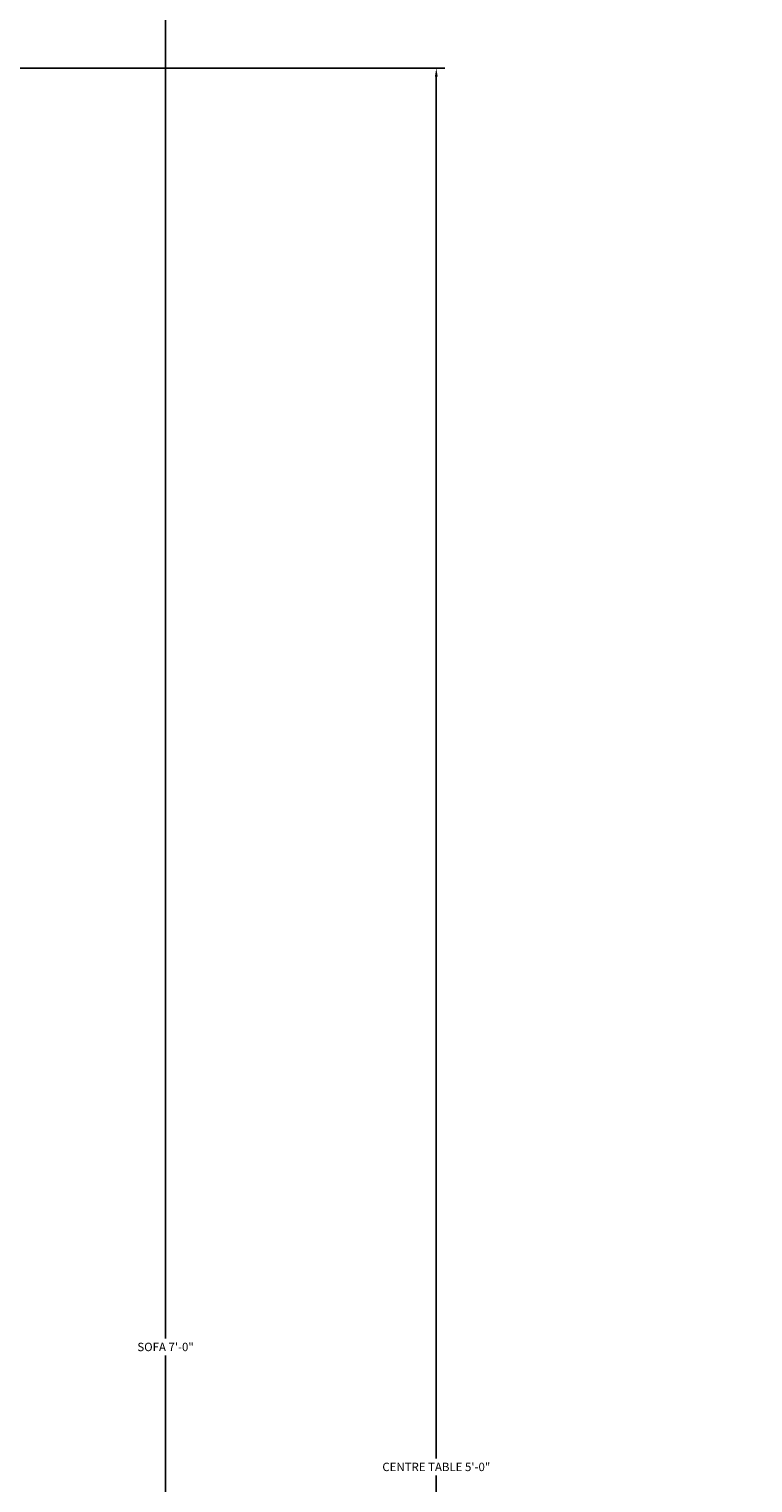
# Model space of a CAD drawing. Units: inches. Extents: x -105 to 1196, y -792 to 119.
# Tile 14 of 23: x 262 to 278, y -349 to -318. Entities that reach past the tile are written whole.
import ezdxf

# ---------------------------------------------------------------- set-up
doc = ezdxf.new("R2010")
doc.units = ezdxf.units.IN
doc.header["$MEASUREMENT"] = 0
doc.layers.add('A-ANNO-DIMS', color=2, linetype='Continuous', lineweight=18)
doc.styles.get("Standard").update_dxf_attribs({"font": 'arial.ttf'})
doc.dimstyles.get("Standard").update_dxf_attribs({"dimtxt": 0.18, "dimasz": 0.18, "dimexe": 0.18, "dimexo": 0.0625, "dimgap": 0.09, "dimtad": 0, "dimtih": 1, "dimtoh": 1, "dimdec": 1, "dimzin": 0, "dimdsep": 46, "dimlunit": 4, "dimtxsty": 'Standard', "dimcen": 0.09, "dimadec": 0, "dimazin": 0, "dimtfac": 1, "dimtdec": 1, "dimtofl": 0, "dimtmove": 0, "dimatfit": 3, "dimfxl": 1, "dimtolj": 1, "dimtzin": 0, "dimarcsym": 0})

# ---------------------------------------------------------------- blocks, each defined once
blk = doc.blocks.new('*D77')
at = {"layer": 'A-ANNO-DIMS', "color": 0, "lineweight": -2, "transparency": 16777216}
for p, q in [((277.544, -304.122), (264.827, -304.122)), ((265.007, -304.302), (265.007, -345.939)), ((265.007, -387.942), (265.007, -346.305)), ((277.544, -388.122), (264.827, -388.122))]:
    blk.add_line(p, q, dxfattribs=at)
at = {"layer": 'A-ANNO-DIMS', "color": 0, "transparency": 16777216}
for points in [[(264.977, -304.302), (265.037, -304.302), (265.007, -304.122)], [(264.977, -387.942), (265.037, -387.942), (265.007, -388.122)]]:
    blk.add_solid(points, dxfattribs=at)
at = {"layer": 'Defpoints', "color": 0, "transparency": 16777216}
for p in [(277.607, -304.122), (265.007, -388.122), (277.607, -388.122)]:
    blk.add_point(p, dxfattribs=at)
at = {"layer": 'A-ANNO-DIMS', "color": 0, "transparency": 16777216, "insert": (265.007, -346.122), "char_height": 0.18, "attachment_point": 5}
blk.add_mtext('\\A1;SOFA 7\'-0"', dxfattribs=at)
blk = doc.blocks.new('*D83')
at = {"layer": 'A-ANNO-DIMS', "color": 0, "lineweight": -2, "transparency": 16777216}
for p, q in [((261.878, -318.695), (270.995, -318.695)), ((270.815, -318.875), (270.815, -348.512)), ((270.815, -378.515), (270.815, -348.878)), ((261.878, -378.695), (270.995, -378.695))]:
    blk.add_line(p, q, dxfattribs=at)
at = {"layer": 'A-ANNO-DIMS', "color": 0, "transparency": 16777216}
for points in [[(270.785, -318.875), (270.845, -318.875), (270.815, -318.695)], [(270.785, -378.515), (270.845, -378.515), (270.815, -378.695)]]:
    blk.add_solid(points, dxfattribs=at)
at = {"layer": 'Defpoints', "color": 0, "transparency": 16777216}
for p in [(261.815, -318.695), (270.815, -318.695), (261.815, -378.695)]:
    blk.add_point(p, dxfattribs=at)
at = {"layer": 'A-ANNO-DIMS', "color": 0, "transparency": 16777216, "insert": (270.815, -348.695), "char_height": 0.18, "attachment_point": 5}
blk.add_mtext('\\A1;CENTRE TABLE 5\'-0"', dxfattribs=at)

msp = doc.modelspace()

# ---------------------------------------------------------------- dimensions: what is measured, and where the dimension line sits
at = {"layer": 'A-ANNO-DIMS'}
for base, p1, p2, angle, text, picture, middle in [((265.007, -388.122), (277.607, -304.122), (277.607, -388.122), 270, 'SOFA <>', '*D77', (265.007, -346.122)), ((270.815, -318.695), (261.815, -378.695), (261.815, -318.695), 90, 'CENTRE TABLE <>', '*D83', (270.815, -348.695))]:
    dim = msp.add_linear_dim(base=base, p1=p1, p2=p2, angle=angle, text=text, dimstyle='Standard', override={"dimdec": 1, "dimlfac": 1, "dimrnd": 0, "dimzin": 1, "dimdsep": 46, "dimlunit": 4, "dimfrac": 2}, dxfattribs=at)
    dim.commit()
    dim.dimension.update_dxf_attribs({"geometry": picture, "text_midpoint": middle})

doc.saveas('drawing.dxf')
